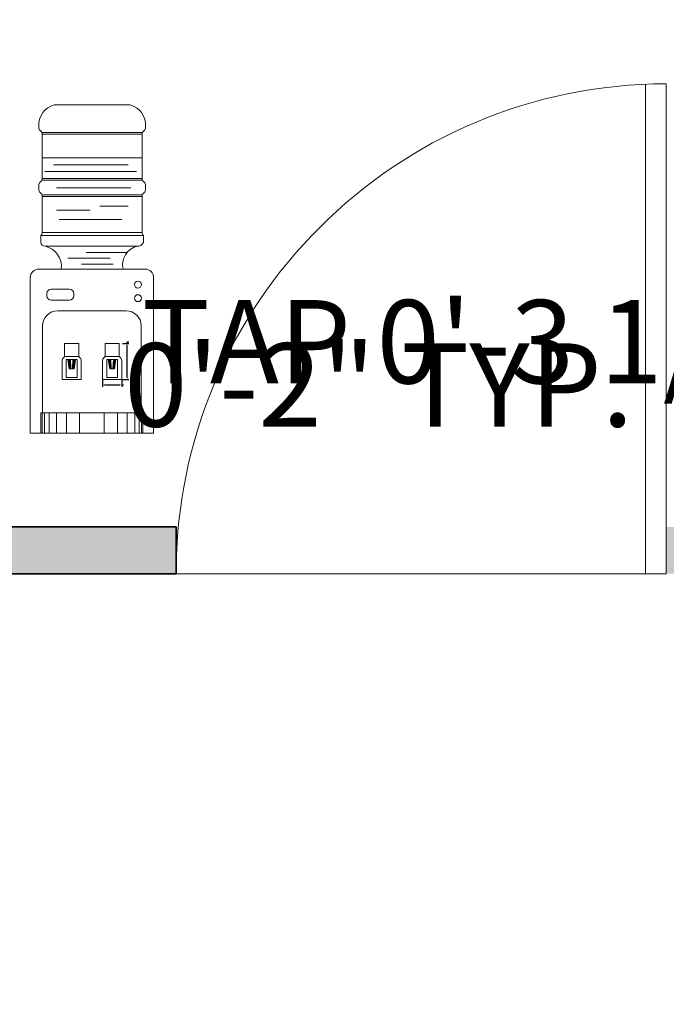
# Model space of a CAD drawing. Units: inches. Extents: x 638 to 1303, y 1 to 699.
# Tile 18 of 21: x 964 to 1026, y 503 to 597. Entities that reach past the tile are written whole.
import ezdxf

# ---------------------------------------------------------------- set-up
doc = ezdxf.new("R2010")
doc.units = ezdxf.units.IN
doc.header["$MEASUREMENT"] = 0
for name, color, linetype, lineweight in [('A-ANNO-DIMS', 2, 'Continuous', 18), ('A-DOOR', 4, 'Continuous', 18), ('A-EQPM', 8, 'Continuous', 15), ('A-WALL', 7, 'Continuous', 35)]:
    doc.layers.add(name, color=color, linetype=linetype, lineweight=lineweight)
doc.layers.add('A-WALL-PATT', color=143, linetype='Continuous', lineweight=13, true_color=0x7aafdf)
doc.styles.get("Standard").update_dxf_attribs({"font": 'arial.ttf'})
doc.dimstyles.get("Standard").update_dxf_attribs({"dimtxt": 8, "dimasz": 0.18, "dimexe": 0.18, "dimexo": 0.0625, "dimgap": 0.09, "dimtad": 0, "dimtih": 1, "dimtoh": 1, "dimdec": 4, "dimzin": 0, "dimdsep": 46, "dimlunit": 3, "dimtxsty": 'Standard', "dimcen": 0.09, "dimadec": 0, "dimazin": 0, "dimtfac": 1, "dimtdec": 4, "dimtofl": 0, "dimtmove": 0, "dimatfit": 3, "dimfxl": 1, "dimtolj": 1, "dimtzin": 0, "dimarcsym": 0})

# ---------------------------------------------------------------- blocks, each defined once
blk = doc.blocks.new('DOOR-SWING-47')
for p, q in [((45, 0), (45, 46.957)), ((47, 0), (47, 47)), ((0, 0), (47, 0))]:
    blk.add_line(p, q)
blk.add_arc((47, 0), 47, 90, 180)
blk = doc.blocks.new('DISPENSER-TAP')
for p, q in [((1.593, 3.447), (0.24, 3.447)), ((0.24, 3.447), (0.24, 2.196)), ((1.593, 2.196), (1.593, 3.447)), ((0.24, 2.196), (0.154, 2.124)), ((0.24, 2.196), (1.593, 2.196)), ((0.396, 0.202), (0.396, 1.917)), ((0.396, 1.917), (1.436, 1.917)), ((0.549, 1.917), (0.683, 1.04)), ((0.582, 1.917), (0.695, 1.04)), ((0.622, 1.917), (0.721, 1.04)), ((0.707, 1.917), (0.773, 1.04)), ((0.796, 1.917), (0.836, 1.04)), ((1.037, 1.917), (0.997, 1.04)), ((1.126, 1.917), (1.06, 1.04)), ((1.21, 1.917), (1.112, 1.04)), ((1.25, 1.917), (1.138, 1.04)), ((1.283, 1.917), (1.149, 1.04)), ((1.436, 1.917), (1.436, 0.202)), ((1.678, 2.124), (1.593, 2.196)), ((0, 1.792), (0, 0)), ((1.149, 1.04), (0.683, 1.04)), ((1.833, 0), (1.833, 1.792)), ((0, 0), (1.833, 0)), ((1.436, 0.202), (0.396, 0.202))]:
    blk.add_line(p, q)
for centre, start, end in [((0.433, 1.792), 130.01999, 180), ((1.4, 1.792), 360, 49.98001)]:
    blk.add_arc(centre, 0.434, start, end)
blk = doc.blocks.new('*D40')
at = {"layer": 'A-ANNO-DIMS', "color": 0, "lineweight": -2, "transparency": 16777216}
for p, q in [((974.203, 566.401), (974.837, 566.401)), ((974.657, 566.401), (974.657, 566.581)), ((974.657, 566.581), (974.837, 566.581)), ((974.657, 563.134), (974.657, 566.221)), ((974.203, 562.954), (974.837, 562.954))]:
    blk.add_line(p, q, dxfattribs=at)
at = {"layer": 'A-ANNO-DIMS', "color": 0, "transparency": 16777216}
for points in [[(974.627, 566.221), (974.687, 566.221), (974.657, 566.401)], [(974.627, 563.134), (974.687, 563.134), (974.657, 562.954)]]:
    blk.add_solid(points, dxfattribs=at)
at = {"layer": 'Defpoints', "color": 0, "transparency": 16777216}
for p in [(974.14, 566.401), (974.657, 566.401), (974.14, 562.954)]:
    blk.add_point(p, dxfattribs=at)
at = {"layer": 'A-ANNO-DIMS', "color": 0, "transparency": 16777216, "insert": (1021.151, 566.581), "char_height": 8, "attachment_point": 5}
blk.add_mtext('\\A1;TAP 0\'-3 1/2" TYP.', dxfattribs=at)
blk = doc.blocks.new('*D41')
at = {"layer": 'A-ANNO-DIMS', "color": 0, "lineweight": -2, "transparency": 16777216}
for p, q in [((972.307, 562.892), (972.307, 562.257)), ((972.487, 562.437), (973.96, 562.437)), ((974.14, 562.892), (974.14, 562.257)), ((974.14, 562.437), (974.32, 562.437))]:
    blk.add_line(p, q, dxfattribs=at)
at = {"layer": 'A-ANNO-DIMS', "color": 0, "transparency": 16777216}
for points in [[(972.487, 562.467), (972.487, 562.407), (972.307, 562.437)], [(973.96, 562.467), (973.96, 562.407), (974.14, 562.437)]]:
    blk.add_solid(points, dxfattribs=at)
at = {"layer": 'Defpoints', "color": 0, "transparency": 16777216}
for p in [(972.307, 562.954), (974.14, 562.954), (974.14, 562.437)]:
    blk.add_point(p, dxfattribs=at)
at = {"layer": 'A-ANNO-DIMS', "color": 0, "transparency": 16777216, "insert": (998.792, 562.437), "char_height": 8, "attachment_point": 5}
blk.add_mtext('\\A1;0\'-2" TYP.', dxfattribs=at)

msp = doc.modelspace()

# ---------------------------------------------------------------- hatches: boundary and pattern name
at = {"layer": 'A-WALL-PATT'}
h = msp.add_hatch(color=256, dxfattribs=at)
h.dxf.hatch_style = 1
h.paths.add_polyline_path([(973.34524, 629.81895), (793.35541, 629.81895), (793.35541, 620.81895), (850.23798, 620.81895), (922.23798, 620.81895), (922.23798, 524.81895), (908.94335, 524.81895), (908.94335, 520.31895), (926.73798, 520.31895), (926.73798, 544.31895), (979.3571, 544.31895), (979.3571, 548.81895), (926.73798, 548.81895), (926.73798, 620.81895), (973.34524, 620.81895)])
h.paths.add_polyline_path([(758.35541, 629.81895), (697.23798, 629.81895), (697.23798, 586.77451), (706.23798, 586.77451), (706.23798, 620.81895), (758.35541, 620.81895)])
h.paths.add_polyline_path([(1075.85281, 629.81895), (1003.34524, 629.81895), (1003.34524, 620.81895), (1046.73798, 620.81895), (1046.73798, 560.81895), (1046.73798, 548.81895), (1026.3571, 548.81895), (1026.3571, 544.31895), (1046.73798, 544.31895), (1046.73798, 486.87457), (1051.23798, 486.87457), (1051.23798, 556.31895), (1162.89753, 556.31895), (1162.89753, 560.81895), (1051.23798, 560.81895), (1051.23798, 620.81895), (1075.85281, 620.81895)])
h.paths.add_polyline_path([(1228.23798, 629.81895), (1105.85281, 629.81895), (1105.85281, 620.81895), (1219.23798, 620.81895), (1219.23798, 560.81895), (1197.89753, 560.81895), (1197.89753, 556.31895), (1219.23798, 556.31895), (1219.23798, 498.80084), (1228.23798, 498.80084)])
h.paths.add_polyline_path([(1051.23798, 439.87457), (1046.73798, 439.87457), (1046.73798, 407.81895), (1219.23798, 407.81895), (1219.23798, 381.66175), (1228.23798, 381.66175), (1228.23798, 451.80084), (1219.23798, 451.80084), (1219.23798, 412.31895), (1051.23798, 412.31895)])
h.paths.add_polyline_path([(1228.23798, 346.66175), (1219.23798, 346.66175), (1219.23798, 335.81895), (1046.73798, 335.81895), (1046.73798, 273.56895), (1051.23798, 273.56895), (1051.23798, 331.31895), (1219.23798, 331.31895), (1219.23798, 308.99654), (1228.23798, 308.99654)])
h.paths.add_polyline_path([(1228.23798, 261.99654), (1219.23798, 261.99654), (1219.23798, 211.31895), (1051.23798, 211.31895), (1051.23798, 226.56895), (1046.73798, 226.56895), (1046.73798, 211.31895), (983.84714, 211.31895), (983.84714, 206.81895), (1219.23798, 206.81895), (1219.23798, 166.83987), (1228.23798, 166.83987)])
h.paths.add_polyline_path([(1228.23798, 119.83987), (1219.23798, 119.83987), (1219.23798, 50.81895), (1197.89277, 50.81895), (1197.89277, 41.81895), (1228.23798, 41.81895)])
h.paths.add_polyline_path([(1162.89277, 50.81895), (1069.02949, 50.81895), (1069.02949, 41.81895), (1162.89277, 41.81895)])
h.paths.add_polyline_path([(1010.02949, 50.81895), (941.89631, 50.81895), (917.77455, 50.81895), (917.77455, 41.81895), (941.89631, 41.81895), (1010.02949, 41.81895)])
h.paths.add_polyline_path([(882.77455, 50.81895), (854.73798, 50.81895), (854.73798, 145.50379), (850.23798, 145.50379), (850.23798, 50.81895), (793.49755, 50.81895), (793.49755, 41.81895), (882.77455, 41.81895)])
h.paths.add_polyline_path([(746.49755, 50.81895), (706.23798, 50.81895), (706.23798, 96.57416), (697.23798, 96.57416), (697.23798, 41.81895), (746.49755, 41.81895)])
h.paths.add_polyline_path([(706.23798, 206.81895), (714.01165, 206.81895), (714.01165, 211.31895), (706.23798, 211.31895), (706.23798, 251.21966), (697.23798, 251.21966), (697.23798, 143.57416), (706.23798, 143.57416)])
h.paths.add_polyline_path([(923.84714, 211.31895), (854.73798, 211.31895), (854.73798, 397.8313), (850.23798, 397.8313), (850.23798, 388.31895), (747.9539, 388.31895), (747.9539, 383.81895), (850.23798, 383.81895), (850.23798, 311.81895), (706.23798, 311.81895), (706.23798, 342.78787), (697.23798, 342.78787), (697.23798, 281.21966), (706.23798, 281.21966), (706.23798, 307.31895), (850.23798, 307.31895), (850.23798, 211.31895), (749.01165, 211.31895), (749.01165, 206.81895), (850.23798, 206.81895), (850.23798, 192.50379), (854.73798, 192.50379), (854.73798, 206.81895), (923.84714, 206.81895)])
h.paths.add_polyline_path([(706.23798, 434.70471), (697.23798, 434.70471), (697.23798, 372.78787), (706.23798, 372.78787), (706.23798, 383.81895), (712.9539, 383.81895), (712.9539, 388.31895), (706.23798, 388.31895)])
h.paths.add_polyline_path([(706.23798, 520.31895), (850.23798, 520.31895), (850.23798, 444.8313), (854.73798, 444.8313), (854.73798, 520.31895), (861.94335, 520.31895), (861.94335, 524.81895), (706.23798, 524.81895), (706.23798, 551.77451), (697.23798, 551.77451), (697.23798, 481.70471), (706.23798, 481.70471)])

# ---------------------------------------------------------------- linework, layer by layer
at = {"layer": 'A-EQPM'}
for p, q in [((974.9508, 589.30314), (967.66964, 589.30314)), ((966.19212, 587.30886), (966.19212, 587.13895)), ((966.31825, 586.85016), (966.39631, 586.77783)), ((966.48952, 586.6466), (976.13092, 586.6466)), ((976.3022, 586.85016), (976.22414, 586.77783)), ((976.42832, 587.13895), (976.42832, 587.30886)), ((966.52243, 586.48903), (976.09802, 586.48903)), ((966.52243, 586.48903), (966.52243, 582.23985)), ((976.09802, 582.23985), (976.09802, 586.48903)), ((966.52243, 584.20551), (976.09802, 584.20551)), ((966.77251, 582.90576), (975.54782, 582.90576)), ((967.59962, 583.54453), (974.75213, 583.54453)), ((966.31825, 581.87873), (966.39631, 581.95106)), ((966.48952, 582.08229), (976.09802, 582.08229)), ((976.09802, 582.23985), (966.52243, 582.23985)), ((976.3022, 581.87873), (976.22414, 581.95106)), ((966.19212, 581.58994), (966.19212, 581.17442)), ((966.31825, 580.88563), (966.39631, 580.8133)), ((967.89973, 581.34494), (975.00222, 581.34494)), ((976.3022, 580.88563), (976.22414, 580.8133)), ((976.42832, 581.17442), (976.42832, 581.58994)), ((966.48952, 580.68207), (976.09802, 580.68207)), ((966.52243, 577.06452), (966.52243, 580.52451)), ((976.09802, 580.52451), (966.52243, 580.52451)), ((976.09802, 580.52451), (976.09802, 577.06452)), ((967.89973, 579.19535), (971.10085, 579.19535)), ((972.05118, 579.59528), (974.75213, 579.59528)), ((968.14982, 578.29552), (974.15192, 578.29552)), ((966.3982, 576.12542), (966.39631, 576.77573)), ((966.39631, 576.77573), (976.22414, 576.77573)), ((966.52243, 577.06452), (976.09802, 577.06452)), ((976.22422, 576.08764), (976.22414, 576.77573)), ((966.79179, 575.74075), (975.60884, 575.74075)), ((968.98662, 574.59547), (973.02748, 574.59547)), ((970.74021, 575.12889), (974.70482, 575.12889)), ((976.37698, 573.55514), (966.19212, 573.55514)), ((970.28275, 574.02396), (973.33245, 574.02396)), ((965.37905, 572.74207), (965.37905, 557.80714)), ((977.19005, 557.80714), (977.19005, 572.74207)), ((967.38496, 571.62738), (969.12114, 571.62738)), ((966.95127, 570.99353), (966.95127, 571.19369)), ((969.12114, 570.55983), (967.38496, 570.55983)), ((969.55483, 571.19369), (969.55483, 570.99353)), ((974.55947, 569.55162), (968.00963, 569.55162)), ((966.56015, 568.10214), (966.56015, 559.77564)), ((976.00895, 559.77564), (976.00895, 568.10214)), ((966.39945, 557.80714), (966.39945, 559.77564)), ((966.39945, 559.77564), (976.16966, 559.77564)), ((966.51986, 557.80714), (966.51986, 559.77564)), ((966.74732, 557.80714), (966.74732, 559.77564)), ((967.17547, 557.80714), (967.17547, 559.77564)), ((967.89798, 557.80714), (967.89798, 559.77564)), ((968.83457, 557.80714), (968.83457, 559.77564)), ((970.10566, 557.80714), (970.10566, 559.77564)), ((972.46345, 557.80714), (972.46345, 559.77564)), ((973.73454, 557.80714), (973.73454, 559.77564)), ((974.67112, 557.80714), (974.67112, 559.77564)), ((975.39363, 557.80714), (975.39363, 559.77564)), ((975.82179, 557.80714), (975.82179, 559.77564)), ((976.04925, 557.80714), (976.04925, 559.77564)), ((976.16966, 559.77564), (976.16966, 557.80714)), ((965.37905, 557.80714), (977.19005, 557.80714)), ((976.16966, 557.80714), (966.39945, 557.80714))]:
    msp.add_line(p, q, dxfattribs=at)
for centre in [(975.69656, 572.06108), (975.69656, 570.76)]:
    msp.add_circle(centre, 0.33361, dxfattribs=at)
for centre, radius, start, end in [((968.18674, 587.37556), 1.99573, 105.0167672, 181.9152145), ((974.4337, 587.37556), 1.99573, 358.0847855, 74.9832328), ((966.58582, 587.13895), 0.3937, 180, 227.1836572), ((966.12873, 586.48903), 0.3937, 0, 47.1836572), ((976.49172, 586.48903), 0.3937, 132.8163428, 180), ((976.03462, 587.13895), 0.3937, 312.8163428, 0), ((966.58582, 581.58994), 0.3937, 132.8163428, 180), ((966.12873, 582.23985), 0.3937, 312.8163428, 0), ((976.49172, 582.23985), 0.3937, 180, 227.1836572), ((976.03462, 581.58994), 0.3937, 0, 47.1836572), ((966.58582, 581.17442), 0.3937, 180, 227.1836572), ((976.03462, 581.17442), 0.3937, 312.8163428, 0), ((966.12873, 580.52451), 0.3937, 0, 47.1836572), ((976.49172, 580.52451), 0.3937, 132.8163428, 180), ((966.12873, 577.06452), 0.3937, 312.8163428, 0), ((976.49172, 577.06452), 0.3937, 180, 227.1836572), ((966.79179, 576.13445), 0.3937, 181.3137415, 270), ((966.37275, 573.79605), 1.98934, 353.0444135, 77.8398817), ((976.06411, 573.96145), 1.83662, 104.3526007, 192.7811742), ((975.6709, 576.34994), 0.61234, 264.1827192, 334.6374952), ((966.19212, 572.74207), 0.81307, 90, 180), ((976.37698, 572.74207), 0.81307, 0, 90), ((967.38496, 571.19369), 0.43369, 90, 180), ((969.12114, 571.19369), 0.43369, 360, 90), ((967.38496, 570.99353), 0.43369, 180, 270), ((969.12114, 570.99353), 0.43369, 270, 0), ((968.00963, 568.10214), 1.44948, 90, 180), ((974.55947, 568.10214), 1.44948, 0, 90)]:
    msp.add_arc(centre, radius, start, end, dxfattribs=at)
at = {"layer": 'A-WALL'}
for p, q in [((979.3571, 548.81895), (926.73798, 548.81895)), ((979.3571, 548.81895), (979.3571, 544.31895)), ((979.3571, 544.31895), (926.73798, 544.31895))]:
    msp.add_line(p, q, dxfattribs=at)

# ---------------------------------------------------------------- block references
at = {"layer": 'A-DOOR'}
msp.add_blockref('DOOR-SWING-47', (979.35675, 544.319), dxfattribs=at)
at = {"layer": 'A-EQPM'}
for p in [(968.4293, 562.954), (972.307, 562.954)]:
    msp.add_blockref('DISPENSER-TAP', p, dxfattribs=at)

# ---------------------------------------------------------------- texts
at = {"layer": 'A-EQPM', "flags": 9}
for tag, p, s in [('YSIZE', (971.28455, 569.55162), '810.6226'), ('XSIZE', (971.28455, 569.55162), '314.5432'), ('ZSIZE', (971.28455, 569.55162), '0.0425'), ('YSIZE', (965.37905, 557.80714), '800.0000'), ('XSIZE', (965.37905, 557.80714), '300.0000'), ('ZSIZE', (965.37905, 557.80714), '0.0000')]:
    msp.add_attdef(tag, p, s, height=0.019685, dxfattribs=at)

# ---------------------------------------------------------------- dimensions: what is measured, and where the dimension line sits
at = {"layer": 'A-ANNO-DIMS'}
dim = msp.add_linear_dim(base=(974.65728, 566.40113), p1=(974.14026, 562.95435), p2=(974.14026, 566.40113), angle=90, text='TAP <> TYP.', dimstyle='Standard', override={"dimdec": 1, "dimlfac": 1, "dimrnd": 0, "dimzin": 1, "dimdsep": 46, "dimlunit": 4, "dimfrac": 2}, dxfattribs=at)
dim.commit()
dim.dimension.update_dxf_attribs({"geometry": '*D40', "text_midpoint": (1021.15102, 566.58113)})
dim = msp.add_linear_dim(base=(974.14026, 562.43734), p1=(972.30655, 562.95435), p2=(974.14026, 562.95435), text='<> TYP.', dimstyle='Standard', override={"dimdec": 1, "dimlfac": 1, "dimrnd": 0, "dimzin": 1, "dimdsep": 46, "dimlunit": 4, "dimfrac": 2}, dxfattribs=at)
dim.commit()
dim.dimension.update_dxf_attribs({"geometry": '*D41', "text_midpoint": (998.79225, 562.43734)})

doc.saveas('drawing.dxf')
